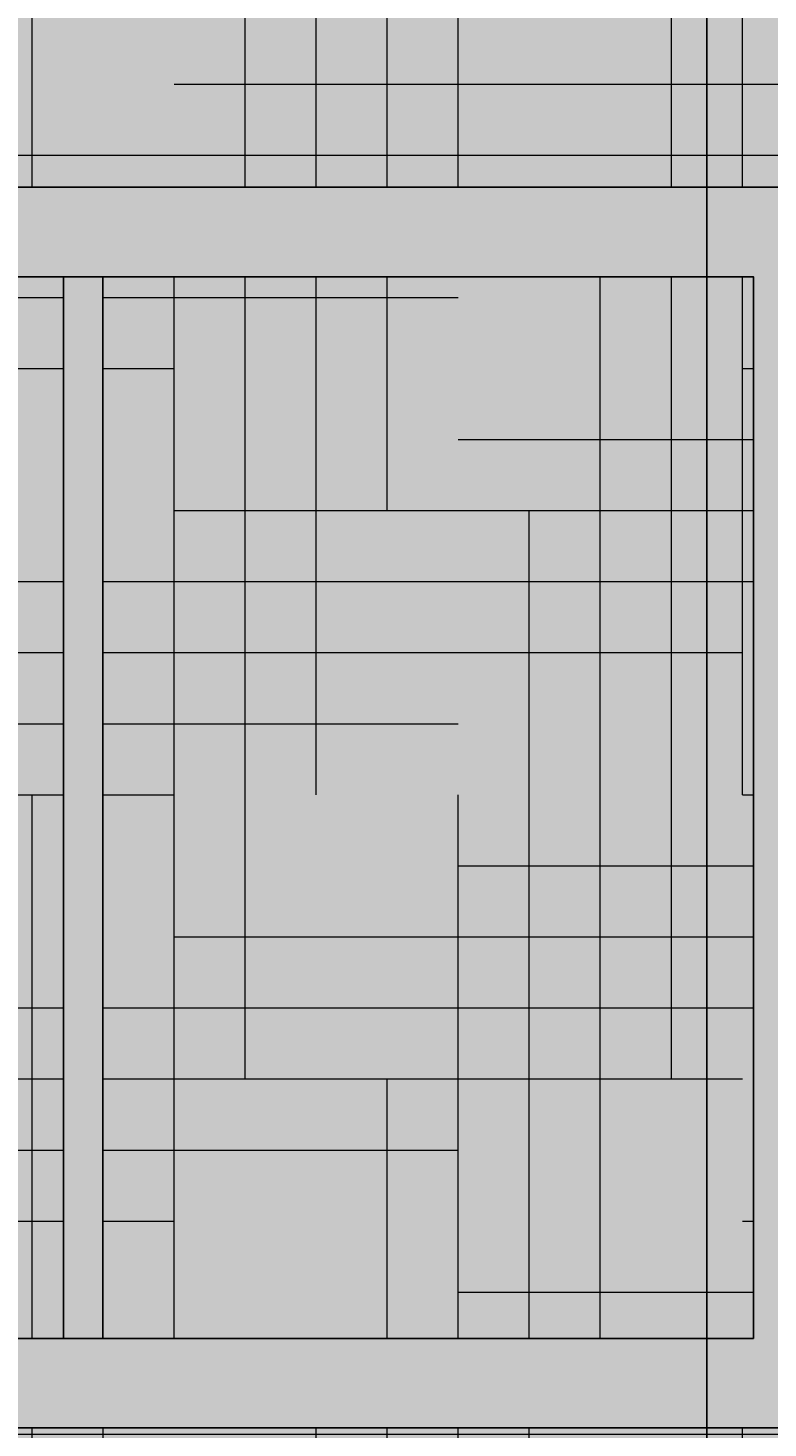
# Model space of a CAD drawing. Units: feet. Extents: x 2695 to 2912, y 795 to 1139.
# Tile 12 of 83: x 2740 to 2756, y 875 to 906. Entities that reach past the tile are written whole.
import ezdxf

# ---------------------------------------------------------------- set-up
doc = ezdxf.new("R2010")
doc.units = ezdxf.units.FT
for name, color, linetype, lineweight in [('A-ANNO-DIMS', 2, 'Continuous', 18), ('A-ELEV-PATT', 252, 'Continuous', 13), ('A-GLAZ', 4, 'Continuous', 25), ('A-GLAZ-PATT', 254, 'Continuous', 13)]:
    doc.layers.add(name, color=color, linetype=linetype, lineweight=lineweight)
doc.styles.get("Standard").update_dxf_attribs({"font": 'arial.ttf'})
doc.dimstyles.get("Standard").update_dxf_attribs({"dimtxt": 0.18, "dimasz": 0.18, "dimexe": 0.18, "dimexo": 0.0625, "dimgap": 0.09, "dimtad": 0, "dimtih": 1, "dimtoh": 1, "dimdec": 1, "dimzin": 0, "dimdsep": 46, "dimlunit": 3, "dimtxsty": 'Standard', "dimcen": 0.09, "dimadec": 0, "dimazin": 0, "dimtfac": 1, "dimtdec": 1, "dimtofl": 0, "dimtmove": 0, "dimatfit": 3, "dimfxl": 1, "dimtolj": 1, "dimtzin": 0, "dimarcsym": 0})

# ---------------------------------------------------------------- blocks, each defined once
blk = doc.blocks.new('*D24')
at = {"layer": 'A-ANNO-DIMS', "color": 0, "lineweight": -2, "transparency": 16777216}
for p, q in [((2730.708, 936.868), (2730.708, 794.976)), ((2755.112, 936.868), (2755.112, 794.976)), ((2730.888, 795.156), (2742.446, 795.156)), ((2754.932, 795.156), (2743.375, 795.156))]:
    blk.add_line(p, q, dxfattribs=at)
at = {"layer": 'A-ANNO-DIMS', "color": 0, "transparency": 16777216}
for points in [[(2730.888, 795.186), (2730.888, 795.126), (2730.708, 795.156)], [(2754.932, 795.186), (2754.932, 795.126), (2755.112, 795.156)]]:
    blk.add_solid(points, dxfattribs=at)
at = {"layer": 'Defpoints', "color": 0, "transparency": 16777216}
for p in [(2730.708, 936.931), (2755.112, 936.931), (2755.112, 795.156)]:
    blk.add_point(p, dxfattribs=at)
at = {"layer": 'A-ANNO-DIMS', "color": 0, "transparency": 16777216, "insert": (2742.91, 795.156), "char_height": 0.18, "attachment_point": 5}
blk.add_mtext('\\A1;24.404', dxfattribs=at)
blk = doc.blocks.new('*D25')
at = {"layer": 'A-ANNO-DIMS', "color": 0, "lineweight": -2, "transparency": 16777216}
for p, q in [((2755.112, 936.868), (2755.112, 794.976)), ((2770.636, 936.868), (2770.636, 794.976)), ((2755.292, 795.156), (2762.419, 795.156)), ((2770.456, 795.156), (2763.329, 795.156))]:
    blk.add_line(p, q, dxfattribs=at)
at = {"layer": 'A-ANNO-DIMS', "color": 0, "transparency": 16777216}
for points in [[(2755.292, 795.186), (2755.292, 795.126), (2755.112, 795.156)], [(2770.456, 795.186), (2770.456, 795.126), (2770.636, 795.156)]]:
    blk.add_solid(points, dxfattribs=at)
at = {"layer": 'Defpoints', "color": 0, "transparency": 16777216}
for p in [(2755.112, 936.931), (2770.636, 936.931), (2770.636, 795.156)]:
    blk.add_point(p, dxfattribs=at)
at = {"layer": 'A-ANNO-DIMS', "color": 0, "transparency": 16777216, "insert": (2762.874, 795.156), "char_height": 0.18, "attachment_point": 5}
blk.add_mtext('\\A1;15.524', dxfattribs=at)

msp = doc.modelspace()

# ---------------------------------------------------------------- hatches: boundary and pattern name
at = {"layer": 'A-ELEV-PATT'}
h = msp.add_hatch(color=256, dxfattribs=at)
h.set_gradient(color2=(0, 0, 0), tint=1)
h.paths.add_polyline_path([(2772.5216, 971.9673), (2770.6361, 971.9673), (2770.6361, 970.7156), (2772.5216, 970.7156)])
h.paths.add_polyline_path([(2773.2702, 971.9673), (2772.5216, 971.9673), (2772.5216, 970.7156), (2773.2702, 970.7156)])
h.paths.add_polyline_path([(2778.0341, 971.9673), (2773.2702, 971.9673), (2773.2702, 970.7156), (2778.0341, 970.7156)])
h.paths.add_polyline_path([(2780.0341, 971.9673), (2778.0341, 971.9673), (2778.0341, 970.7156), (2780.0341, 970.7156)])
h.paths.add_polyline_path([(2841.575, 971.9673), (2780.0341, 971.9673), (2780.0341, 970.7156), (2841.575, 970.7156)])
h.paths.add_polyline_path([(2843.575, 971.9673), (2841.575, 971.9673), (2841.575, 970.7156), (2843.575, 970.7156)])
h.paths.add_polyline_path([(2888.1882, 971.9673), (2843.575, 971.9673), (2843.575, 970.7156), (2888.1882, 970.7156)])
h.paths.add_polyline_path([(2888.9368, 971.9673), (2888.1882, 971.9673), (2888.1882, 970.7156), (2888.9368, 970.7156)], flags=17)
h.paths.add_polyline_path([(2890.6361, 971.9673), (2888.9368, 971.9673), (2888.9368, 970.7156), (2890.6361, 970.7156)])
h.paths.add_polyline_path([(2888.9368, 971.9673), (2888.1882, 971.9673), (2888.1882, 964.8267), (2888.9368, 964.8267)])
h.paths.add_polyline_path([(2888.9368, 964.8267), (2888.1882, 964.8267), (2888.1882, 964.1328), (2888.9368, 964.1328)])
h.paths.add_polyline_path([(2890.6361, 964.8267), (2888.9368, 964.8267), (2888.9368, 964.1328), (2890.6361, 964.1328)])
h.paths.add_polyline_path([(2888.1882, 964.8267), (2770.6361, 964.8267), (2770.6361, 964.1328), (2888.1882, 964.1328)])
h.paths.add_polyline_path([(2888.9368, 964.1328), (2888.1882, 964.1328), (2888.1882, 936.9306), (2888.9368, 936.9306)])
h.paths.add_polyline_path([(2890.6361, 956.614), (2888.9368, 956.614), (2888.9368, 955.9202), (2890.6361, 955.9202)])
h.paths.add_polyline_path([(2888.1882, 956.614), (2770.6361, 956.614), (2770.6361, 955.9202), (2888.1882, 955.9202)])
h.paths.add_polyline_path([(2890.6361, 949.2892), (2888.9368, 949.2892), (2888.9368, 948.5954), (2890.6361, 948.5954)])
h.paths.add_polyline_path([(2888.1882, 949.2892), (2770.6361, 949.2892), (2770.6361, 948.5954), (2888.1882, 948.5954)])
h.paths.add_polyline_path([(2890.6361, 941.3507), (2888.9368, 941.3507), (2888.9368, 940.6569), (2890.6361, 940.6569)])
h.paths.add_polyline_path([(2888.1882, 941.3507), (2770.6361, 941.3507), (2770.6361, 940.6569), (2888.1882, 940.6569)])
h.paths.add_polyline_path([(2773.2702, 970.7156), (2772.5216, 970.7156), (2772.5216, 964.8267), (2773.2702, 964.8267)])
h.paths.add_polyline_path([(2773.2702, 964.1328), (2772.5216, 964.1328), (2772.5216, 956.614), (2773.2702, 956.614)])
h.paths.add_polyline_path([(2773.2702, 955.9202), (2772.5216, 955.9202), (2772.5216, 936.9306), (2773.2702, 936.9306)])
h.paths.add_polyline_path([(2810.7893, 970.7156), (2810.0407, 970.7156), (2810.0407, 964.8267), (2810.7893, 964.8267)], flags=17)
h.paths.add_polyline_path([(2810.7893, 964.1328), (2810.0407, 964.1328), (2810.0407, 956.614), (2810.7893, 956.614)], flags=17)
h.paths.add_polyline_path([(2810.7893, 955.9202), (2810.0407, 955.9202), (2810.0407, 949.2892), (2810.7893, 949.2892)], flags=17)
h.paths.add_polyline_path([(2810.7893, 971.9673), (2810.0407, 971.9673), (2810.0407, 941.3507), (2810.7893, 941.3507)])
h.paths.add_polyline_path([(2810.7893, 940.6569), (2810.0407, 940.6569), (2810.0407, 936.9306), (2810.7893, 936.9306)])
h.paths.add_polyline_path([(2780.0341, 1018.8235), (2841.575, 1018.8235), (2841.575, 971.9673), (2843.575, 971.9673), (2843.575, 1020.8235), (2778.0341, 1020.8235), (2778.0341, 971.9673), (2780.0341, 971.9673)])
h.paths.add_polyline_path([(2780.0341, 970.7156), (2778.0341, 970.7156), (2778.0341, 964.8267), (2780.0341, 964.8267)])
h.paths.add_polyline_path([(2780.0341, 964.1328), (2778.0341, 964.1328), (2778.0341, 956.614), (2780.0341, 956.614)])
h.paths.add_polyline_path([(2780.0341, 955.9202), (2778.0341, 955.9202), (2778.0341, 949.2892), (2780.0341, 949.2892)])
h.paths.add_polyline_path([(2780.0341, 948.5954), (2778.0341, 948.5954), (2778.0341, 941.3507), (2780.0341, 941.3507)])
h.paths.add_polyline_path([(2780.0341, 940.6569), (2778.0341, 940.6569), (2778.0341, 936.9306), (2780.0341, 936.9306)])
h.paths.add_polyline_path([(2843.575, 940.6569), (2841.575, 940.6569), (2841.575, 936.9306), (2843.575, 936.9306)])
h.paths.add_polyline_path([(2843.575, 948.5954), (2841.575, 948.5954), (2841.575, 941.3507), (2843.575, 941.3507)])
h.paths.add_polyline_path([(2843.575, 970.7156), (2841.575, 970.7156), (2841.575, 964.8267), (2843.575, 964.8267)])
h.paths.add_polyline_path([(2843.575, 964.1328), (2841.575, 964.1328), (2841.575, 956.614), (2843.575, 956.614)])
h.paths.add_polyline_path([(2843.575, 955.9202), (2841.575, 955.9202), (2841.575, 949.2892), (2843.575, 949.2892)])
h.paths.add_polyline_path([(2805.0538, 874.1057), (2803.9681, 874.1057), (2803.9681, 846.2857), (2805.0538, 846.2857)])
h.paths.add_polyline_path([(2758.1515, 902.577), (2724.1893, 902.577), (2724.1893, 874.8571), (2758.1515, 874.8571)])
h.paths.add_polyline_path([(2726.1893, 900.577), (2756.1515, 900.577), (2756.1515, 876.8571), (2726.1893, 876.8571)], flags=16)
h.paths.add_polyline_path([(2740.7302, 900.577), (2741.6105, 900.577), (2741.6105, 876.8571), (2740.7302, 876.8571)], flags=0)
h = msp.add_hatch(color=256, dxfattribs=at)
h.set_gradient(color1=(255, 255, 255))
h.paths.add_polyline_path([(2770.6361, 924.3105), (2716.5358, 924.3105), (2716.5358, 810.9306), (2770.6361, 810.9306)])
h.paths.add_polyline_path([(2758.1515, 902.577), (2758.1515, 874.8571), (2724.1893, 874.8571), (2724.1893, 902.577)], flags=16)
h.paths.add_polyline_path([(2756.1515, 900.577), (2756.1515, 876.8571), (2726.1893, 876.8571), (2726.1893, 900.577)], flags=0)
h.paths.add_polyline_path([(2740.7302, 900.577), (2741.6105, 900.577), (2741.6105, 876.8571), (2740.7302, 876.8571)], flags=0)
h = msp.add_hatch(dxfattribs=at)
h.set_pattern_fill('HOUND', color=256, style=0)
h.paths.add_polyline_path([(2770.6361, 924.3105), (2716.5358, 924.3105), (2716.5358, 810.9306), (2770.6361, 810.9306)])
h.paths.add_polyline_path([(2724.1893, 874.8571), (2724.1893, 902.577), (2758.1515, 902.577), (2758.1515, 874.8571)], flags=16)
h.paths.add_polyline_path([(2756.1515, 876.8571), (2726.1893, 876.8571), (2726.1893, 900.577), (2756.1515, 900.577)], flags=0)
h.paths.add_polyline_path([(2741.6105, 876.8571), (2740.7302, 876.8571), (2740.7302, 900.577), (2741.6105, 900.577)], flags=0)
at = {"layer": 'A-GLAZ-PATT'}
h = msp.add_hatch(color=256, dxfattribs=at)
h.set_gradient(color1=(153, 185, 219), color2=(153, 185, 219))
h.paths.add_polyline_path([(2740.7302, 900.577), (2726.1893, 900.577), (2726.1893, 876.8571), (2740.7302, 876.8571)])
h.paths.add_polyline_path([(2756.1515, 900.577), (2741.6105, 900.577), (2741.6105, 876.8571), (2756.1515, 876.8571)])
h = msp.add_hatch(color=256, dxfattribs=at)
h.set_gradient(color1=(153, 185, 219), color2=(153, 185, 219))
h.paths.add_polyline_path([(2740.7302, 900.577), (2726.1893, 900.577), (2726.1893, 876.8571), (2740.7302, 876.8571)])
h.paths.add_polyline_path([(2756.1515, 900.577), (2741.6105, 900.577), (2741.6105, 876.8571), (2756.1515, 876.8571)])

# ---------------------------------------------------------------- linework, layer by layer
at = {"layer": 'A-GLAZ'}
for p, q in [((2724.1893, 902.577), (2758.1515, 902.577)), ((2758.1515, 874.8571), (2724.1893, 874.8571))]:
    msp.add_line(p, q, dxfattribs=at)
for points in [[(2724.1893, 902.577), (2758.1515, 902.577), (2758.1515, 874.8571), (2724.1893, 874.8571)], [(2726.1893, 900.577), (2756.1515, 900.577), (2756.1515, 876.8571), (2726.1893, 876.8571)], [(2726.1893, 900.577), (2756.1515, 900.577), (2756.1515, 876.8571), (2726.1893, 876.8571)], [(2740.7302, 900.577), (2741.6105, 900.577), (2741.6105, 876.8571), (2740.7302, 876.8571)]]:
    msp.add_lwpolyline(points, close=True, dxfattribs=at)

# ---------------------------------------------------------------- dimensions: what is measured, and where the dimension line sits
at = {"layer": 'A-ANNO-DIMS'}
for base, p1, p2, picture, middle in [((2755.1125, 795.1556), (2730.7081, 936.9306), (2755.1125, 936.9306), '*D24', (2742.9103, 795.1556)), ((2770.6361, 795.1556), (2755.1125, 936.9306), (2770.6361, 936.9306), '*D25', (2762.8743, 795.1556))]:
    dim = msp.add_linear_dim(base=base, p1=p1, p2=p2, dimstyle='Standard', override={"dimdec": 3, "dimlfac": 1, "dimrnd": 0, "dimzin": 0, "dimdsep": 46, "dimlunit": 2}, dxfattribs=at)
    dim.commit()
    dim.dimension.update_dxf_attribs({"geometry": picture, "text_midpoint": middle})

doc.saveas('drawing.dxf')
